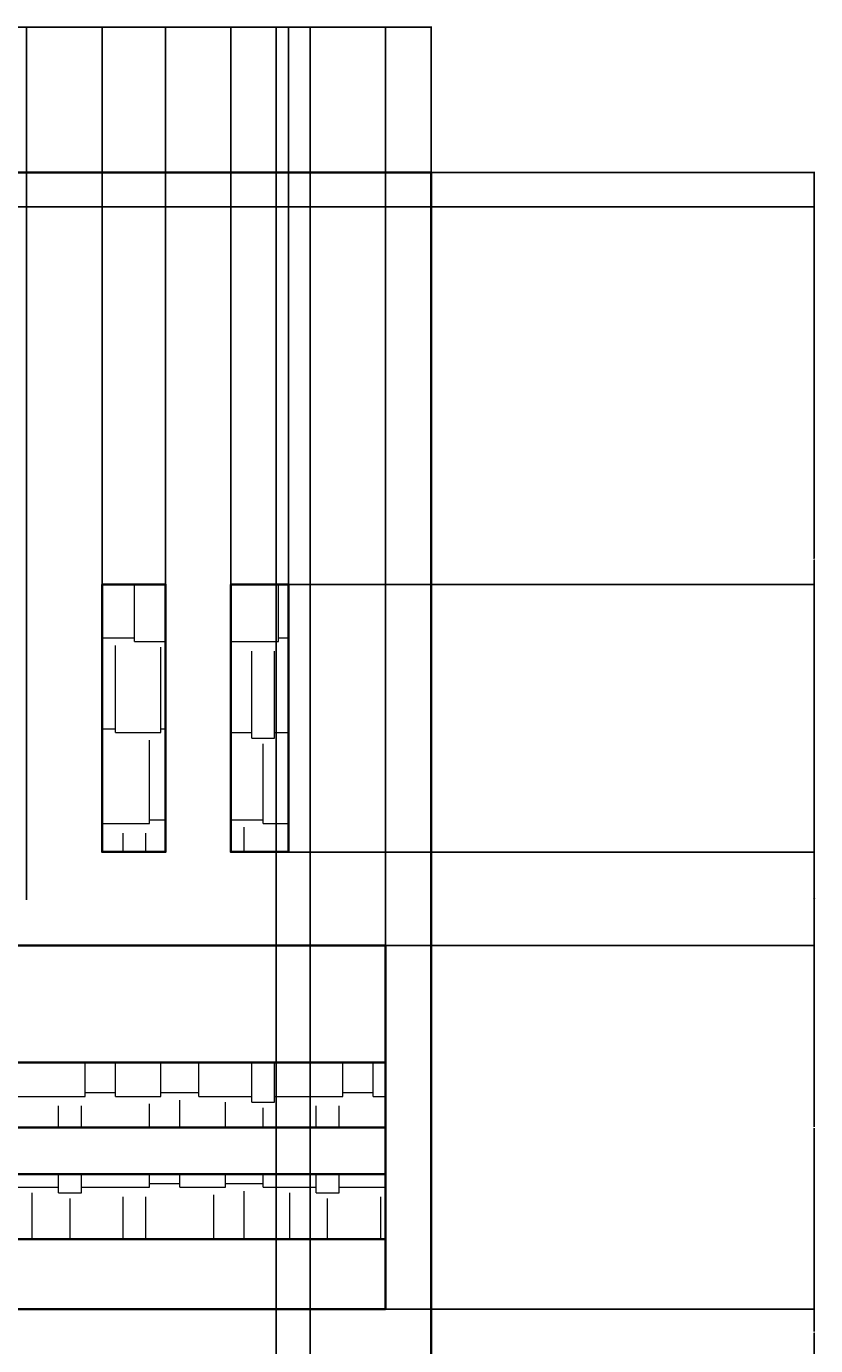
# Model space of a CAD drawing. Units: inches. Extents: x -15 to 605, y -220 to 570.
# Tile 10 of 10: x 397 to 605, y 222 to 570. Entities that reach past the tile are written whole.
import ezdxf

# ---------------------------------------------------------------- set-up
doc = ezdxf.new("R2010")
doc.units = ezdxf.units.IN
doc.header["$MEASUREMENT"] = 0
for name, color, linetype, lineweight in [('A-ANNO-DIMS', 2, 'Continuous', 18), ('A-ELEV', 7, 'Continuous', 35), ('A-ELEV-PATT', 8, 'Continuous', 13)]:
    doc.layers.add(name, color=color, linetype=linetype, lineweight=lineweight)
doc.styles.get("Standard").update_dxf_attribs({"font": 'arial.ttf'})
doc.dimstyles.get("Standard").update_dxf_attribs({"dimtxt": 0.18, "dimasz": 0.18, "dimexe": 0.18, "dimexo": 0.0625, "dimgap": 0.09, "dimtad": 0, "dimtih": 1, "dimtoh": 1, "dimdec": 4, "dimzin": 0, "dimdsep": 46, "dimtxsty": 'Standard', "dimcen": 0.09, "dimadec": 0, "dimazin": 0, "dimtfac": 1, "dimtdec": 4, "dimtofl": 0, "dimtmove": 0, "dimatfit": 3, "dimfxl": 1, "dimtolj": 1, "dimtzin": 0, "dimarcsym": 0})

# ---------------------------------------------------------------- blocks, each defined once
blk = doc.blocks.new('*D8')
at = {"layer": 'A-ANNO-DIMS', "color": 0, "lineweight": -2, "transparency": 16777216}
for p, q in [((23.99, 3.88), (23.99, 570.4)), ((24.17, 570.22), (263.7, 570.22)), ((503.81, 570.22), (264.28, 570.22)), ((503.99, 531.88), (503.99, 570.4))]:
    blk.add_line(p, q, dxfattribs=at)
at = {"layer": 'A-ANNO-DIMS', "color": 0, "transparency": 16777216}
for points in [[(24.17, 570.25), (24.17, 570.19), (23.99, 570.22)], [(503.81, 570.25), (503.81, 570.19), (503.99, 570.22)]]:
    blk.add_solid(points, dxfattribs=at)
at = {"layer": 'Defpoints', "color": 0, "transparency": 16777216}
for p in [(503.99, 570.22), (503.99, 531.82), (23.99, 3.82)]:
    blk.add_point(p, dxfattribs=at)
at = {"layer": 'A-ANNO-DIMS', "color": 0, "transparency": 16777216, "insert": (263.99, 570.22), "char_height": 0.18, "attachment_point": 5}
blk.add_mtext('\\A1;480', dxfattribs=at)
blk = doc.blocks.new('*D9')
at = {"layer": 'A-ANNO-DIMS', "color": 0, "lineweight": -2, "transparency": 16777216}
for p, q in [((503.92, 531.82), (-14.59, 531.82)), ((-14.41, 531.64), (-14.41, 208)), ((-14.41, -116), (-14.41, 207.64)), ((23.92, -116.18), (-14.59, -116.18))]:
    blk.add_line(p, q, dxfattribs=at)
at = {"layer": 'A-ANNO-DIMS', "color": 0, "transparency": 16777216}
for points in [[(-14.44, 531.64), (-14.38, 531.64), (-14.41, 531.82)], [(-14.44, -116), (-14.38, -116), (-14.41, -116.18)]]:
    blk.add_solid(points, dxfattribs=at)
at = {"layer": 'Defpoints', "color": 0, "transparency": 16777216}
for p in [(-14.41, 531.82), (503.99, 531.82), (23.99, -116.18)]:
    blk.add_point(p, dxfattribs=at)
at = {"layer": 'A-ANNO-DIMS', "color": 0, "transparency": 16777216, "insert": (-14.41, 207.82), "char_height": 0.18, "attachment_point": 5}
blk.add_mtext('\\A1;648', dxfattribs=at)
blk = doc.blocks.new('*D15')
at = {"layer": 'A-ANNO-DIMS', "color": 0, "lineweight": -2, "transparency": 16777216}
for p, q in [((492.05, 231.82), (605.3, 231.82)), ((605.12, 231.64), (605.12, 226)), ((605.12, 220), (605.12, 225.64)), ((492.05, 219.82), (605.3, 219.82))]:
    blk.add_line(p, q, dxfattribs=at)
at = {"layer": 'A-ANNO-DIMS', "color": 0, "transparency": 16777216}
for points in [[(605.09, 231.64), (605.15, 231.64), (605.12, 231.82)], [(605.09, 220), (605.15, 220), (605.12, 219.82)]]:
    blk.add_solid(points, dxfattribs=at)
at = {"layer": 'Defpoints', "color": 0, "transparency": 16777216}
for p in [(491.99, 231.82), (605.12, 231.82), (491.99, 219.82)]:
    blk.add_point(p, dxfattribs=at)
at = {"layer": 'A-ANNO-DIMS', "color": 0, "transparency": 16777216, "insert": (605.12, 225.82), "char_height": 0.18, "attachment_point": 5}
blk.add_mtext('\\A1;12', dxfattribs=at)
blk = doc.blocks.new('*D16')
at = {"layer": 'A-ANNO-DIMS', "color": 0, "lineweight": -2, "transparency": 16777216}
for p, q in [((492.05, 327.82), (605.3, 327.82)), ((605.12, 327.64), (605.12, 280)), ((605.12, 232), (605.12, 279.64)), ((492.05, 231.82), (605.3, 231.82))]:
    blk.add_line(p, q, dxfattribs=at)
at = {"layer": 'A-ANNO-DIMS', "color": 0, "transparency": 16777216}
for points in [[(605.09, 327.64), (605.15, 327.64), (605.12, 327.82)], [(605.09, 232), (605.15, 232), (605.12, 231.82)]]:
    blk.add_solid(points, dxfattribs=at)
at = {"layer": 'Defpoints', "color": 0, "transparency": 16777216}
for p in [(491.99, 327.82), (605.12, 327.82), (491.99, 231.82)]:
    blk.add_point(p, dxfattribs=at)
at = {"layer": 'A-ANNO-DIMS', "color": 0, "transparency": 16777216, "insert": (605.12, 279.82), "char_height": 0.18, "attachment_point": 5}
blk.add_mtext('\\A1;96', dxfattribs=at)
blk = doc.blocks.new('*D17')
at = {"layer": 'A-ANNO-DIMS', "color": 0, "lineweight": -2, "transparency": 16777216}
for p, q in [((504.05, 531.82), (605.3, 531.82)), ((605.12, 531.64), (605.12, 430)), ((605.12, 328), (605.12, 429.64)), ((492.05, 327.82), (605.3, 327.82))]:
    blk.add_line(p, q, dxfattribs=at)
at = {"layer": 'A-ANNO-DIMS', "color": 0, "transparency": 16777216}
for points in [[(605.09, 531.64), (605.15, 531.64), (605.12, 531.82)], [(605.09, 328), (605.15, 328), (605.12, 327.82)]]:
    blk.add_solid(points, dxfattribs=at)
at = {"layer": 'Defpoints', "color": 0, "transparency": 16777216}
for p in [(503.99, 531.82), (605.12, 531.82), (491.99, 327.82)]:
    blk.add_point(p, dxfattribs=at)
at = {"layer": 'A-ANNO-DIMS', "color": 0, "transparency": 16777216, "insert": (605.12, 429.82), "char_height": 0.18, "attachment_point": 5}
blk.add_mtext('\\A1;204', dxfattribs=at)
blk = doc.blocks.new('*D20')
at = {"layer": 'A-ANNO-DIMS', "color": 0, "lineweight": -2, "transparency": 16777216}
for p, q in [((332.99, 435.88), (332.99, 570.4)), ((333.17, 570.22), (418.22, 570.22)), ((503.81, 570.22), (418.75, 570.22)), ((503.99, 531.88), (503.99, 570.4))]:
    blk.add_line(p, q, dxfattribs=at)
at = {"layer": 'A-ANNO-DIMS', "color": 0, "transparency": 16777216}
for points in [[(333.17, 570.25), (333.17, 570.19), (332.99, 570.22)], [(503.81, 570.25), (503.81, 570.19), (503.99, 570.22)]]:
    blk.add_solid(points, dxfattribs=at)
at = {"layer": 'Defpoints', "color": 0, "transparency": 16777216}
for p in [(503.99, 570.22), (503.99, 531.82), (332.99, 435.82)]:
    blk.add_point(p, dxfattribs=at)
at = {"layer": 'A-ANNO-DIMS', "color": 0, "transparency": 16777216, "insert": (418.49, 570.22), "char_height": 0.18, "attachment_point": 5}
blk.add_mtext('\\A1;171', dxfattribs=at)
blk = doc.blocks.new('*D58')
at = {"layer": 'A-ANNO-DIMS', "color": 0, "lineweight": -2, "transparency": 16777216}
for p, q in [((376.71, -44.82), (376.71, 570.4)), ((376.89, 570.22), (419.58, 570.22)), ((462.92, 570.22), (420.23, 570.22)), ((463.1, -45.87), (463.1, 570.4))]:
    blk.add_line(p, q, dxfattribs=at)
at = {"layer": 'A-ANNO-DIMS', "color": 0, "transparency": 16777216}
for points in [[(376.89, 570.25), (376.89, 570.19), (376.71, 570.22)], [(462.92, 570.25), (462.92, 570.19), (463.1, 570.22)]]:
    blk.add_solid(points, dxfattribs=at)
at = {"layer": 'Defpoints', "color": 0, "transparency": 16777216}
for p in [(463.1, 570.22), (376.71, -44.88), (463.1, -45.94)]:
    blk.add_point(p, dxfattribs=at)
at = {"layer": 'A-ANNO-DIMS', "color": 0, "transparency": 16777216, "insert": (419.9, 570.22), "char_height": 0.18, "attachment_point": 5}
blk.add_mtext('\\A1;86.4', dxfattribs=at)
blk = doc.blocks.new('*D59')
at = {"layer": 'A-ANNO-DIMS', "color": 0, "lineweight": -2, "transparency": 16777216}
for p, q in [((463.1, -45.87), (463.1, 570.4)), ((463.28, 570.22), (467.45, 570.22)), ((471.92, 570.22), (467.75, 570.22)), ((472.1, -45.87), (472.1, 570.4))]:
    blk.add_line(p, q, dxfattribs=at)
at = {"layer": 'A-ANNO-DIMS', "color": 0, "transparency": 16777216}
for points in [[(463.28, 570.25), (463.28, 570.19), (463.1, 570.22)], [(471.92, 570.25), (471.92, 570.19), (472.1, 570.22)]]:
    blk.add_solid(points, dxfattribs=at)
at = {"layer": 'Defpoints', "color": 0, "transparency": 16777216}
for p in [(472.1, 570.22), (463.1, -45.94), (472.1, -45.94)]:
    blk.add_point(p, dxfattribs=at)
at = {"layer": 'A-ANNO-DIMS', "color": 0, "transparency": 16777216, "insert": (467.6, 570.22), "char_height": 0.18, "attachment_point": 5}
blk.add_mtext('\\A1;9', dxfattribs=at)
blk = doc.blocks.new('*D75')
at = {"layer": 'A-ANNO-DIMS', "color": 0, "lineweight": -2, "transparency": 16777216}
for p, q in [((333.05, 531.82), (605.3, 531.82)), ((605.12, 531.64), (605.12, 527.5)), ((605.12, 523), (605.12, 527.14)), ((333.05, 522.82), (605.3, 522.82))]:
    blk.add_line(p, q, dxfattribs=at)
at = {"layer": 'A-ANNO-DIMS', "color": 0, "transparency": 16777216}
for points in [[(605.09, 531.64), (605.15, 531.64), (605.12, 531.82)], [(605.09, 523), (605.15, 523), (605.12, 522.82)]]:
    blk.add_solid(points, dxfattribs=at)
at = {"layer": 'Defpoints', "color": 0, "transparency": 16777216}
for p in [(332.99, 531.82), (605.12, 531.82), (332.99, 522.82)]:
    blk.add_point(p, dxfattribs=at)
at = {"layer": 'A-ANNO-DIMS', "color": 0, "transparency": 16777216, "insert": (605.12, 527.32), "char_height": 0.18, "attachment_point": 5}
blk.add_mtext('\\A1;9', dxfattribs=at)
blk = doc.blocks.new('*D88')
at = {"layer": 'A-ANNO-DIMS', "color": 0, "lineweight": -2, "transparency": 16777216}
for p, q in [((385.19, 351.88), (385.19, 570.4)), ((385.37, 570.22), (390.98, 570.22)), ((397.01, 570.22), (391.4, 570.22)), ((397.19, 339.88), (397.19, 570.4))]:
    blk.add_line(p, q, dxfattribs=at)
at = {"layer": 'A-ANNO-DIMS', "color": 0, "transparency": 16777216}
for points in [[(385.37, 570.25), (385.37, 570.19), (385.19, 570.22)], [(397.01, 570.25), (397.01, 570.19), (397.19, 570.22)]]:
    blk.add_solid(points, dxfattribs=at)
at = {"layer": 'Defpoints', "color": 0, "transparency": 16777216}
for p in [(397.19, 570.22), (385.19, 351.82), (397.19, 339.82)]:
    blk.add_point(p, dxfattribs=at)
at = {"layer": 'A-ANNO-DIMS', "color": 0, "transparency": 16777216, "insert": (391.19, 570.22), "char_height": 0.18, "attachment_point": 5}
blk.add_mtext('\\A1;12', dxfattribs=at)
blk = doc.blocks.new('*D89')
at = {"layer": 'A-ANNO-DIMS', "color": 0, "lineweight": -2, "transparency": 16777216}
for p, q in [((397.19, 339.88), (397.19, 570.4)), ((397.37, 570.22), (406.72, 570.22)), ((416.99, 570.22), (407.64, 570.22)), ((417.17, 352.57), (417.17, 570.4))]:
    blk.add_line(p, q, dxfattribs=at)
at = {"layer": 'A-ANNO-DIMS', "color": 0, "transparency": 16777216}
for points in [[(397.37, 570.25), (397.37, 570.19), (397.19, 570.22)], [(416.99, 570.25), (416.99, 570.19), (417.17, 570.22)]]:
    blk.add_solid(points, dxfattribs=at)
at = {"layer": 'Defpoints', "color": 0, "transparency": 16777216}
for p in [(417.17, 570.22), (417.17, 352.51), (397.19, 339.82)]:
    blk.add_point(p, dxfattribs=at)
at = {"layer": 'A-ANNO-DIMS', "color": 0, "transparency": 16777216, "insert": (407.18, 570.22), "char_height": 0.18, "attachment_point": 5}
blk.add_mtext('\\A1;19.975', dxfattribs=at)
blk = doc.blocks.new('*D90')
at = {"layer": 'A-ANNO-DIMS', "color": 0, "lineweight": -2, "transparency": 16777216}
for p, q in [((417.17, 352.57), (417.17, 570.4)), ((417.35, 570.22), (425.08, 570.22)), ((433.73, 570.22), (425.99, 570.22)), ((433.91, 352.57), (433.91, 570.4))]:
    blk.add_line(p, q, dxfattribs=at)
at = {"layer": 'A-ANNO-DIMS', "color": 0, "transparency": 16777216}
for points in [[(417.35, 570.25), (417.35, 570.19), (417.17, 570.22)], [(433.73, 570.25), (433.73, 570.19), (433.91, 570.22)]]:
    blk.add_solid(points, dxfattribs=at)
at = {"layer": 'Defpoints', "color": 0, "transparency": 16777216}
for p in [(433.91, 570.22), (417.17, 352.51), (433.91, 352.51)]:
    blk.add_point(p, dxfattribs=at)
at = {"layer": 'A-ANNO-DIMS', "color": 0, "transparency": 16777216, "insert": (425.54, 570.22), "char_height": 0.18, "attachment_point": 5}
blk.add_mtext('\\A1;16.743', dxfattribs=at)
blk = doc.blocks.new('*D91')
at = {"layer": 'A-ANNO-DIMS', "color": 0, "lineweight": -2, "transparency": 16777216}
for p, q in [((433.91, 352.57), (433.91, 570.4)), ((434.09, 570.22), (442.07, 570.22)), ((450.96, 570.22), (442.98, 570.22)), ((451.14, 352.57), (451.14, 570.4))]:
    blk.add_line(p, q, dxfattribs=at)
at = {"layer": 'A-ANNO-DIMS', "color": 0, "transparency": 16777216}
for points in [[(434.09, 570.25), (434.09, 570.19), (433.91, 570.22)], [(450.96, 570.25), (450.96, 570.19), (451.14, 570.22)]]:
    blk.add_solid(points, dxfattribs=at)
at = {"layer": 'Defpoints', "color": 0, "transparency": 16777216}
for p in [(451.14, 570.22), (433.91, 352.51), (451.14, 352.51)]:
    blk.add_point(p, dxfattribs=at)
at = {"layer": 'A-ANNO-DIMS', "color": 0, "transparency": 16777216, "insert": (442.53, 570.22), "char_height": 0.18, "attachment_point": 5}
blk.add_mtext('\\A1;17.235', dxfattribs=at)
blk = doc.blocks.new('*D92')
at = {"layer": 'A-ANNO-DIMS', "color": 0, "lineweight": -2, "transparency": 16777216}
for p, q in [((451.14, 352.57), (451.14, 570.4)), ((451.32, 570.22), (458.32, 570.22)), ((466.23, 570.22), (459.23, 570.22)), ((466.41, 352.57), (466.41, 570.4))]:
    blk.add_line(p, q, dxfattribs=at)
at = {"layer": 'A-ANNO-DIMS', "color": 0, "transparency": 16777216}
for points in [[(451.32, 570.25), (451.32, 570.19), (451.14, 570.22)], [(466.23, 570.25), (466.23, 570.19), (466.41, 570.22)]]:
    blk.add_solid(points, dxfattribs=at)
at = {"layer": 'Defpoints', "color": 0, "transparency": 16777216}
for p in [(466.41, 570.22), (451.14, 352.51), (466.41, 352.51)]:
    blk.add_point(p, dxfattribs=at)
at = {"layer": 'A-ANNO-DIMS', "color": 0, "transparency": 16777216, "insert": (458.78, 570.22), "char_height": 0.18, "attachment_point": 5}
blk.add_mtext('\\A1;15.265', dxfattribs=at)
blk = doc.blocks.new('*D93')
at = {"layer": 'A-ANNO-DIMS', "color": 0, "lineweight": -2, "transparency": 16777216}
for p, q in [((466.41, 352.57), (466.41, 570.4)), ((466.59, 570.22), (478.73, 570.22)), ((491.81, 570.22), (479.66, 570.22)), ((491.99, 327.88), (491.99, 570.4))]:
    blk.add_line(p, q, dxfattribs=at)
at = {"layer": 'A-ANNO-DIMS', "color": 0, "transparency": 16777216}
for points in [[(466.59, 570.25), (466.59, 570.19), (466.41, 570.22)], [(491.81, 570.25), (491.81, 570.19), (491.99, 570.22)]]:
    blk.add_solid(points, dxfattribs=at)
at = {"layer": 'Defpoints', "color": 0, "transparency": 16777216}
for p in [(491.99, 570.22), (466.41, 352.51), (491.99, 327.82)]:
    blk.add_point(p, dxfattribs=at)
at = {"layer": 'A-ANNO-DIMS', "color": 0, "transparency": 16777216, "insert": (479.2, 570.22), "char_height": 0.18, "attachment_point": 5}
blk.add_mtext('\\A1;25.577', dxfattribs=at)
blk = doc.blocks.new('*D94')
at = {"layer": 'A-ANNO-DIMS', "color": 0, "lineweight": -2, "transparency": 16777216}
for p, q in [((466.47, 352.51), (605.3, 352.51)), ((605.12, 352.33), (605.12, 340.35)), ((605.12, 328), (605.12, 339.98)), ((492.05, 327.82), (605.3, 327.82))]:
    blk.add_line(p, q, dxfattribs=at)
at = {"layer": 'A-ANNO-DIMS', "color": 0, "transparency": 16777216}
for points in [[(605.09, 352.33), (605.15, 352.33), (605.12, 352.51)], [(605.09, 328), (605.15, 328), (605.12, 327.82)]]:
    blk.add_solid(points, dxfattribs=at)
at = {"layer": 'Defpoints', "color": 0, "transparency": 16777216}
for p in [(466.41, 352.51), (605.12, 352.51), (491.99, 327.82)]:
    blk.add_point(p, dxfattribs=at)
at = {"layer": 'A-ANNO-DIMS', "color": 0, "transparency": 16777216, "insert": (605.12, 340.17), "char_height": 0.18, "attachment_point": 5}
blk.add_mtext('\\A1;24.693', dxfattribs=at)
blk = doc.blocks.new('*D95')
at = {"layer": 'A-ANNO-DIMS', "color": 0, "lineweight": -2, "transparency": 16777216}
for p, q in [((466.47, 423.11), (605.3, 423.11)), ((605.12, 422.93), (605.12, 387.99)), ((605.12, 352.69), (605.12, 387.63)), ((466.47, 352.51), (605.3, 352.51))]:
    blk.add_line(p, q, dxfattribs=at)
at = {"layer": 'A-ANNO-DIMS', "color": 0, "transparency": 16777216}
for points in [[(605.09, 422.93), (605.15, 422.93), (605.12, 423.11)], [(605.09, 352.69), (605.15, 352.69), (605.12, 352.51)]]:
    blk.add_solid(points, dxfattribs=at)
at = {"layer": 'Defpoints', "color": 0, "transparency": 16777216}
for p in [(466.41, 423.11), (605.12, 423.11), (466.41, 352.51)]:
    blk.add_point(p, dxfattribs=at)
at = {"layer": 'A-ANNO-DIMS', "color": 0, "transparency": 16777216, "insert": (605.12, 387.81), "char_height": 0.18, "attachment_point": 5}
blk.add_mtext('\\A1;70.6', dxfattribs=at)

msp = doc.modelspace()

# ---------------------------------------------------------------- hatches: boundary and pattern name
at = {"layer": 'A-ELEV-PATT'}
h = msp.add_hatch(dxfattribs=at)
h.set_pattern_fill('AR-RSHKE', color=256, scale=2)
h.set_pattern_definition([(0, (-191.319, 0), (51, 24), [12, -10, 14, -6, 18, -8]), (0, (-179.319, 1), (51, 24), [10, -38, 8, -12]), (0, (-155.319, -1.5), (51, 24), [6, -62]), (90, (-191.319, 0), (-17, 24), [23, -73]), (90, (-179.319, 0), (-17, 24), [22.5, -73.5]), (90, (-169.319, 0), (-17, 24), [21, -75]), (90, (-155.319, -1.5), (-17, 24), [23, -73]), (90, (-149.319, -1.5), (-17, 24), [23, -73]), (90, (-131.319, 0), (-17, 24), [22, -74])])
h.paths.add_polyline_path([(491.9872, 80.9192), (382.0304, 80.9192), (382.0304, 63.8187), (491.9872, 63.8187)])
h.paths.add_polyline_path([(491.9872, 51.4763), (382.0304, 51.4763), (382.0304, 34.3758), (491.9872, 34.3758)])
h.paths.add_polyline_path([(433.9097, 207.1093), (417.1672, 207.1093), (417.1672, 136.5115), (433.9097, 136.5115)])
h.paths.add_polyline_path([(466.4098, 207.1093), (451.1446, 207.1093), (451.1446, 136.5115), (466.4098, 136.5115)])
h.paths.add_polyline_path([(491.9872, 296.9192), (382.0304, 296.9192), (382.0304, 279.8187), (491.9872, 279.8187)])
h.paths.add_polyline_path([(491.9872, 267.4763), (382.0304, 267.4763), (382.0304, 250.3758), (491.9872, 250.3758)])
h.paths.add_polyline_path([(433.9097, 423.1093), (417.1672, 423.1093), (417.1672, 352.5115), (433.9097, 352.5115)])
h.paths.add_polyline_path([(466.4098, 423.1093), (451.1446, 423.1093), (451.1446, 352.5115), (466.4098, 352.5115)])

# ---------------------------------------------------------------- linework, layer by layer
at = {"layer": 'A-ELEV'}
for p, q in [((263.8163, 531.8187), (503.9872, 531.8187)), ((491.9872, 327.8187), (140.9872, 327.8187)), ((491.9872, 231.8187), (491.9872, 327.8187)), ((491.9872, 231.8187), (140.9872, 231.8187))]:
    msp.add_line(p, q, dxfattribs=at)
msp.add_lwpolyline([(23.9872, 123.8187), (23.9872, 3.8187), (503.9872, 3.8187), (503.9872, 123.8187), (503.9872, 531.8187)], dxfattribs=at)
for points in [[(417.1672, 423.1093), (433.9097, 423.1093), (433.9097, 352.5115), (417.1672, 352.5115)], [(451.1446, 423.1093), (466.4098, 423.1093), (466.4098, 352.5115), (451.1446, 352.5115)], [(491.9872, 279.8187), (382.0304, 279.8187), (382.0304, 296.9192), (491.9872, 296.9192)], [(491.9872, 250.3758), (382.0304, 250.3758), (382.0304, 267.4763), (491.9872, 267.4763)]]:
    msp.add_lwpolyline(points, close=True, dxfattribs=at)

# ---------------------------------------------------------------- dimensions: what is measured, and where the dimension line sits
at = {"layer": 'A-ANNO-DIMS'}
for base, p1, p2, override, picture, middle in [((503.9872, 570.2187), (23.9872, 3.8187), (503.9872, 531.8187), {"dimdec": 0, "dimlfac": 1, "dimrnd": 0, "dimzin": 0, "dimdsep": 46, "dimlunit": 2}, '*D8', (263.9872, 570.2187)), ((503.9872, 570.2187), (332.9872, 435.8187), (503.9872, 531.8187), {"dimdec": 0, "dimlfac": 1, "dimrnd": 0, "dimzin": 0, "dimdsep": 46, "dimlunit": 2}, '*D20', (418.4872, 570.2187)), ((463.1032, 570.2187), (376.7066, -44.8803), (463.1032, -45.9373), {"dimdec": 1, "dimlfac": 1, "dimrnd": 0, "dimzin": 0, "dimdsep": 46, "dimlunit": 2}, '*D58', (419.9049, 570.2187)), ((397.1921, 570.2187), (385.1921, 351.8187), (397.1921, 339.8187), {"dimdec": 0, "dimlfac": 1, "dimrnd": 0, "dimzin": 0, "dimdsep": 46, "dimlunit": 2}, '*D88', (391.1921, 570.2187)), ((417.1672, 570.2187), (397.1921, 339.8187), (417.1672, 352.5115), {"dimdec": 3, "dimlfac": 1, "dimrnd": 0, "dimzin": 0, "dimdsep": 46, "dimlunit": 2}, '*D89', (407.1797, 570.2187)), ((433.909701, 570.218732), (417.167199, 352.511486), (433.909701, 352.511486), {"dimdec": 3, "dimlfac": 1, "dimrnd": 0, "dimzin": 0, "dimdsep": 46, "dimlunit": 2}, '*D90', (425.53845, 570.218732)), ((451.1446, 570.2187), (433.9097, 352.5115), (451.1446, 352.5115), {"dimdec": 3, "dimlfac": 1, "dimrnd": 0, "dimzin": 0, "dimdsep": 46, "dimlunit": 2}, '*D91', (442.5272, 570.2187)), ((466.4098, 570.2187), (451.1446, 352.5115), (466.4098, 352.5115), {"dimdec": 3, "dimlfac": 1, "dimrnd": 0, "dimzin": 0, "dimdsep": 46, "dimlunit": 2}, '*D92', (458.7772, 570.2187)), ((472.1032, 570.2187), (463.1032, -45.9373), (472.1032, -45.9373), {"dimdec": 0, "dimlfac": 1, "dimrnd": 0, "dimzin": 0, "dimdsep": 46, "dimlunit": 2}, '*D59', (467.6032, 570.2187)), ((491.9872, 570.2187), (466.4098, 352.5115), (491.9872, 327.8187), {"dimdec": 3, "dimlfac": 1, "dimrnd": 0, "dimzin": 0, "dimdsep": 46, "dimlunit": 2}, '*D93', (479.1985, 570.2187))]:
    dim = msp.add_linear_dim(base=base, p1=p1, p2=p2, dimstyle='Standard', override=override, dxfattribs=at)
    dim.commit()
    dim.dimension.update_dxf_attribs({"geometry": picture, "text_midpoint": middle})
for base, p1, p2, override, picture, middle in [((-14.4128, 531.8187), (23.9872, -116.1813), (503.9872, 531.8187), {"dimdec": 0, "dimlfac": 1, "dimrnd": 0, "dimzin": 0, "dimdsep": 46, "dimlunit": 2}, '*D9', (-14.4128, 207.8187)), ((605.1161, 531.8187), (332.9872, 522.8187), (332.9872, 531.8187), {"dimdec": 0, "dimlfac": 1, "dimrnd": 0, "dimzin": 0, "dimdsep": 46, "dimlunit": 2}, '*D75', (605.1161, 527.3187)), ((605.1161, 531.8187), (491.9872, 327.8187), (503.9872, 531.8187), {"dimdec": 0, "dimlfac": 1, "dimrnd": 0, "dimzin": 0, "dimdsep": 46, "dimlunit": 2}, '*D17', (605.1161, 429.8187)), ((605.1161, 423.1093), (466.4098, 352.5115), (466.4098, 423.1093), {"dimdec": 1, "dimlfac": 1, "dimrnd": 0, "dimzin": 0, "dimdsep": 46, "dimlunit": 2}, '*D95', (605.1161, 387.8104)), ((605.1161, 352.5115), (491.9872, 327.8187), (466.4098, 352.5115), {"dimdec": 3, "dimlfac": 1, "dimrnd": 0, "dimzin": 0, "dimdsep": 46, "dimlunit": 2}, '*D94', (605.1161, 340.1651)), ((605.1161, 327.8187), (491.9872, 231.8187), (491.9872, 327.8187), {"dimdec": 0, "dimlfac": 1, "dimrnd": 0, "dimzin": 0, "dimdsep": 46, "dimlunit": 2}, '*D16', (605.1161, 279.8187)), ((605.1161, 231.8187), (491.9872, 219.8187), (491.9872, 231.8187), {"dimdec": 0, "dimlfac": 1, "dimrnd": 0, "dimzin": 0, "dimdsep": 46, "dimlunit": 2}, '*D15', (605.1161, 225.8187))]:
    dim = msp.add_linear_dim(base=base, p1=p1, p2=p2, angle=90, dimstyle='Standard', override=override, dxfattribs=at)
    dim.commit()
    dim.dimension.update_dxf_attribs({"geometry": picture, "text_midpoint": middle})

doc.saveas('drawing.dxf')
